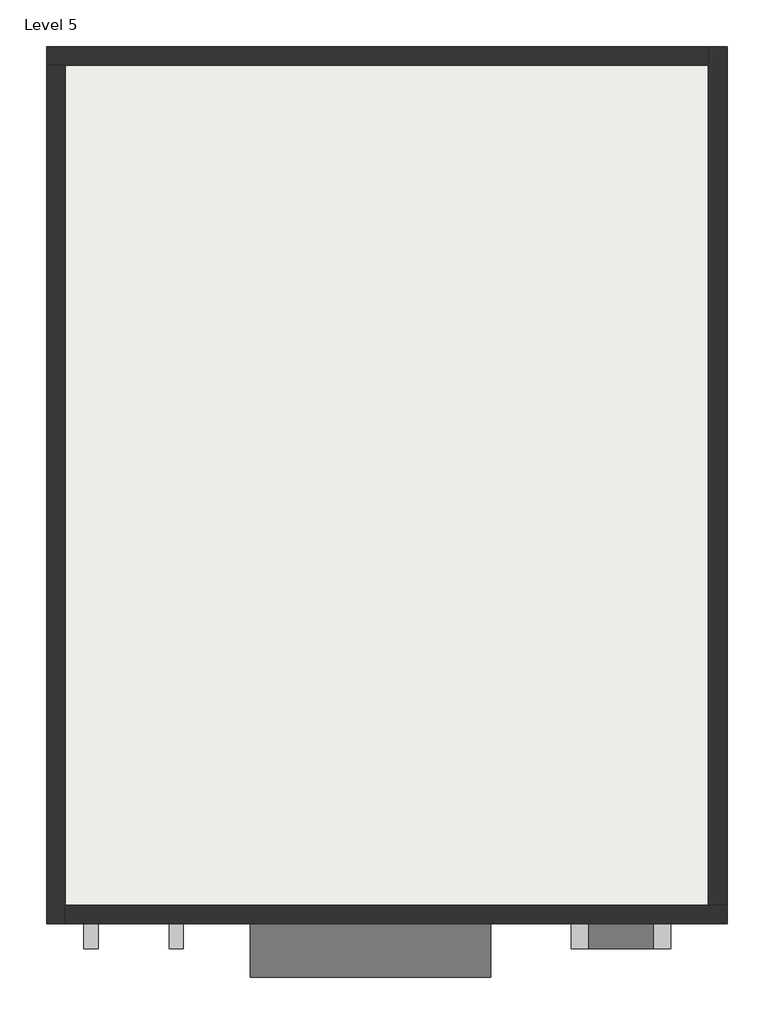
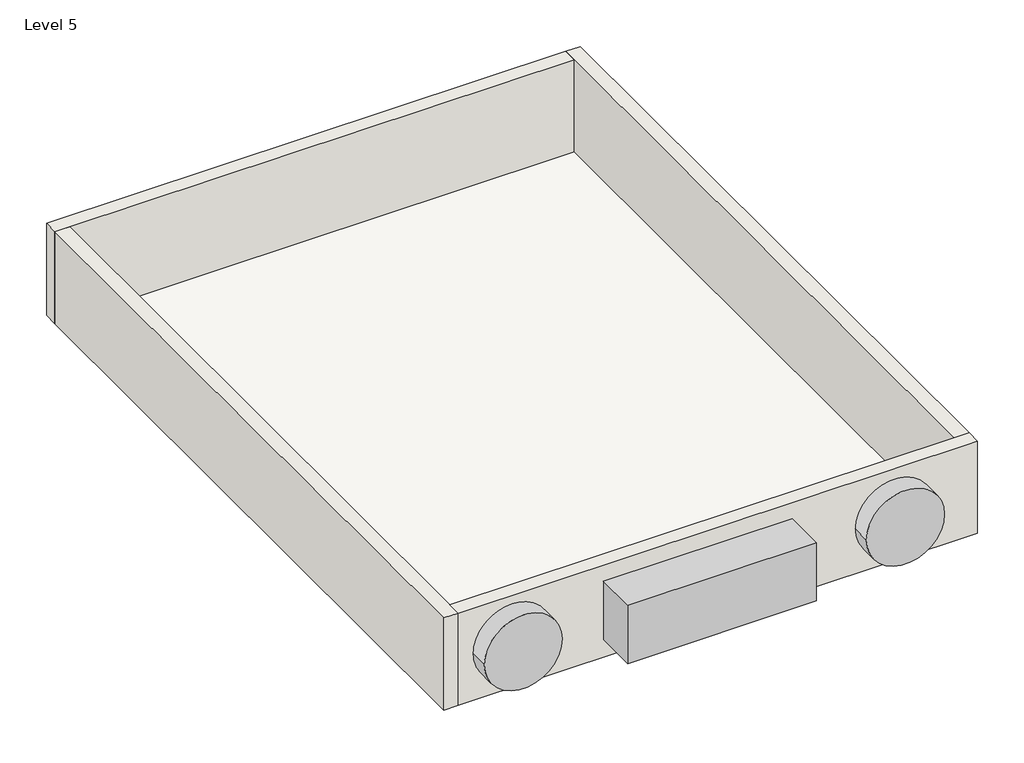
# One storey: 4 walls, 1 proxy, 1 roof.
"""IFC4 building model written with IfcOpenShell, lengths in millimetres."""

from ifc_helpers import new_model, si_unit, frame, origin, place, context, project, spatial, polyline, outline, extrude, faceted_brep, transform, mapped, element, save
from components import generic_models_1_generic_models_1_f32fedec

model = new_model("IFC4")

# Units and contexts
model_context = context("Model", 3, world=origin())
ifc_project = project(units=[si_unit("LENGTHUNIT", "METRE", prefix="MILLI")], contexts=[model_context])

# Site, building, storey
site = spatial("IfcSite", under=ifc_project)
building = spatial("IfcBuilding", under=site)
storey = spatial("IfcBuildingStorey", under=building, Name="Level 5", Elevation=9601.2)

# Proxy
placement = place(None, origin())
generic_models_1_generic_models_1_shape = generic_models_1_generic_models_1_f32fedec(model_context)
element("IfcBuildingElementProxy", 1, Name="Generic Models 1 : Generic Models 1", ObjectType="Generic Models 1 : Generic Models 1", at=placement, inside=storey, context=model_context, shape_type="MappedRepresentation", body=[
    mapped(generic_models_1_generic_models_1_shape, transform((0.0, 0.0, 0.0), x_axis=(1.0, 0.0, 0.0), y_axis=(0.0, 1.0, 0.0), z_axis=(0.0, 0.0, 1.0))),
])

# Roof
element("IfcRoof", 2, ObjectType="Generic - 12\"", at=placement, inside=storey, context=model_context, shape_type="SweptSolid", body=[
    extrude(outline(polyline([(-5198.5915084, 5688.0435985), (2688.1084916, 5688.0435985), (2688.1084916, -4611.6564015), (-5198.5915084, -4611.6564015), (-5198.5915084, 5688.0435985)])), frame((0.0, 0.0, 9448.8), z_axis=(0.0, 0.0, 1.0), x_axis=(1.0, 0.0, 0.0)), (0.0, 0.0, 1.0), 152.4),
])

# Walls
element("IfcWall", 3, ObjectType="WALL9\"", at=placement, inside=storey, context=model_context, shape_type="Brep", body=[
    faceted_brep([(-5427.1915084, 5688.0435985, 9601.2), (-5198.5915084, 5688.0435985, 9601.2), (2688.1084916, 5688.0435985, 9601.2), (2688.1084916, 5688.0435985, 11125.2), (-5198.5915084, 5688.0435985, 11125.2), (-5427.1915084, 5688.0435985, 11125.2), (-5427.1915084, 5916.6435985, 9601.2), (-5427.1915084, 5916.6435985, 11125.2), (2688.1084916, 5916.6435985, 11125.2), (2688.1084916, 5916.6435985, 9601.2)], [[[0, 1, 2, 3, 4, 5]], [[6, 7, 8, 9]], [[2, 1, 0, 6, 9]], [[5, 4, 3, 8, 7]], [[0, 5, 7, 6]], [[3, 2, 9, 8]]]),
])
element("IfcWall", 4, ObjectType="WALL9\"", at=placement, inside=storey, context=model_context, shape_type="Brep", body=[
    faceted_brep([(-5198.5915084, -4840.2564015, 9601.2), (-5198.5915084, -4611.6564015, 9601.2), (-5198.5915084, 5688.0435985, 9601.2), (-5198.5915084, 5688.0435985, 11125.2), (-5198.5915084, -4611.6564015, 11125.2), (-5198.5915084, -4840.2564015, 11125.2), (-5427.1915084, -4840.2564015, 9601.2), (-5427.1915084, -4840.2564015, 11125.2), (-5427.1915084, 5688.0435985, 11125.2), (-5427.1915084, 5688.0435985, 9601.2)], [[[0, 1, 2, 3, 4, 5]], [[6, 7, 8, 9]], [[2, 1, 0, 6, 9]], [[5, 4, 3, 8, 7]], [[0, 5, 7, 6]], [[3, 2, 9, 8]]]),
])
element("IfcWall", 5, ObjectType="WALL9\"", at=placement, inside=storey, context=model_context, shape_type="Brep", body=[
    faceted_brep([(2916.7084916, -4611.6564015, 9601.2), (2688.1084916, -4611.6564015, 9601.2), (-5198.5915084, -4611.6564015, 9601.2), (-5198.5915084, -4611.6564015, 11125.2), (2688.1084916, -4611.6564015, 11125.2), (2916.7084916, -4611.6564015, 11125.2), (2916.7084916, -4840.2564015, 9601.2), (2916.7084916, -4840.2564015, 11125.2), (-5198.5915084, -4840.2564015, 11125.2), (-5198.5915084, -4840.2564015, 9601.2)], [[[0, 1, 2, 3, 4, 5]], [[6, 7, 8, 9]], [[2, 1, 0, 6, 9]], [[5, 4, 3, 8, 7]], [[0, 5, 7, 6]], [[3, 2, 9, 8]]]),
])
element("IfcWall", 6, ObjectType="WALL9\"", at=placement, inside=storey, context=model_context, shape_type="Brep", body=[
    faceted_brep([(2688.1084916, 5916.6435985, 9601.2), (2688.1084916, 5688.0435985, 9601.2), (2688.1084916, -4611.6564015, 9601.2), (2688.1084916, -4611.6564015, 11125.2), (2688.1084916, 5688.0435985, 11125.2), (2688.1084916, 5916.6435985, 11125.2), (2916.7084916, 5916.6435985, 9601.2), (2916.7084916, 5916.6435985, 11125.2), (2916.7084916, -4611.6564015, 11125.2), (2916.7084916, -4611.6564015, 9601.2)], [[[0, 1, 2, 3, 4, 5]], [[6, 7, 8, 9]], [[2, 1, 0, 6, 9]], [[5, 4, 3, 8, 7]], [[0, 5, 7, 6]], [[3, 2, 9, 8]]]),
])

save(model, "model.ifc")

# Revit data of these elements
# Type "Generic - 12\""
#   Assembly Code = "B1020"
#   Layers, outside or top first: 0' - 6" no material (function 1)
# Type "WALL9\""
#   Assembly Code = "B2010"
#   Layers, outside or top first: 0' - 9" no material (function 1)
# Element 1 (IfcBuildingElementProxy, "Generic Models 1 : Generic Models 1")
#   Phase Created = New Construction
#   Materials on its faces: "Parking Stripe", "Brick, Common"
# Element 2 (IfcRoof, "Generic - 12\"")
#   built-in parameter 1001705 = 31.5 (stored number, unit not read)
#   built-in parameter 1001701 = -0.5 (stored number, unit not read)
#   built-in parameter 1001710 = 33615
#   Phase Created = New Construction
#   Materials on its faces: "Default Roof"
# Elements 3, 4, 5, 6 (IfcWall, "WALL9\"")
#   Top Offset = 0' - 0"
#   Base Offset = 0' - 0"
#   Unconnected Height = 5' - 0"
#   wall height = 5' - 0"
#   Phase Created = New Construction
#   Base Constraint = Level 5
#   Materials on its faces: "Default Wall", "Carpet (1)"
# Materials
#   "Parking Stripe": class "Paint", colour RGB 250 250 91, transparency 0, Cost = 0
#   "Brick, Common": class "Masonry", colour RGB 170 98 104, transparency 0, Description = "Common brick", Cost = 0
#   "Default Roof": colour RGB 88 101 114, transparency 0, Cost = 0
#   "Default Wall": colour RGB 128 128 128, transparency 0, Cost = 0
#   "Carpet (1)": class "Carpet", colour RGB 124 80 67, transparency 0, Description = "Interior finish", Cost = 0
